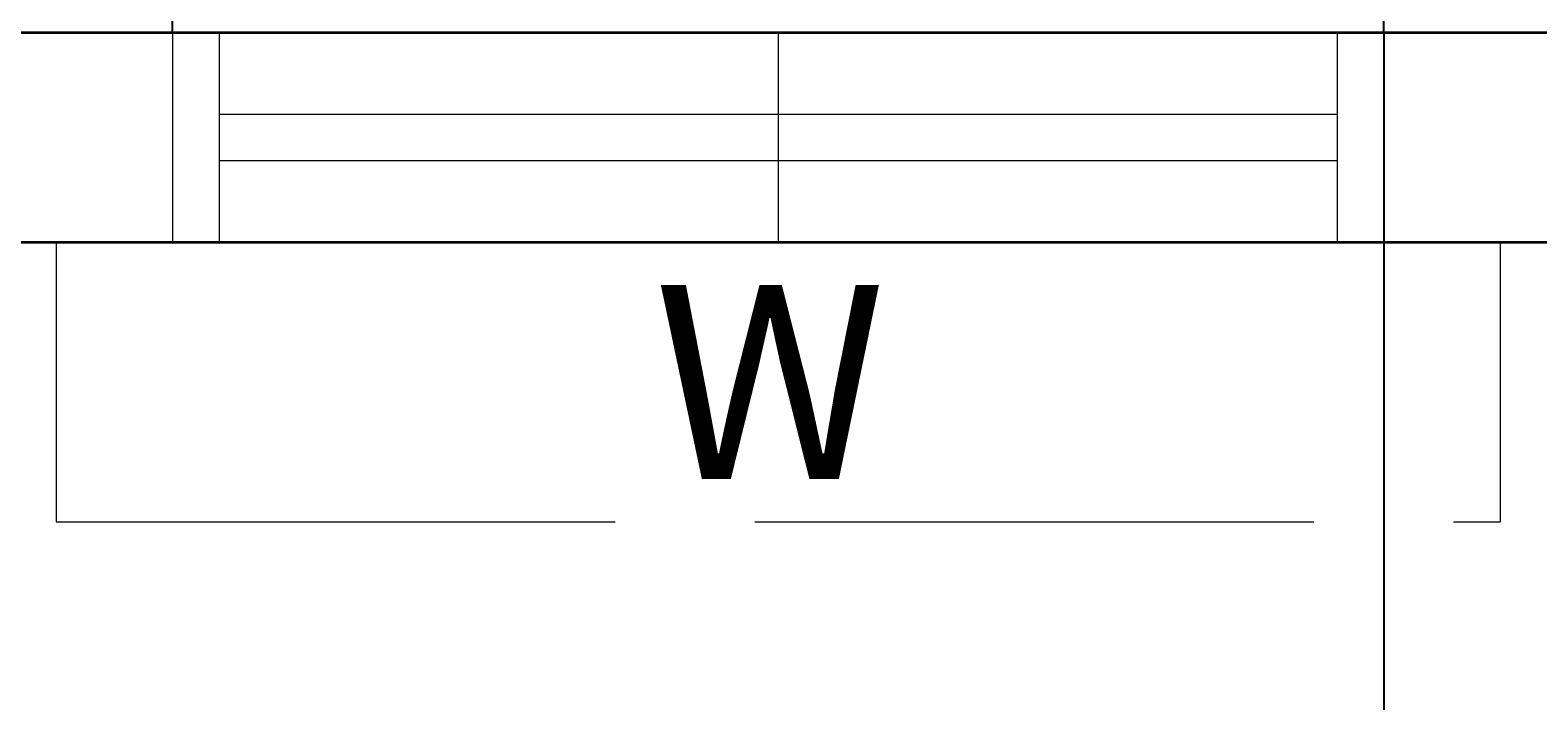
# Model space of a CAD drawing. Units: inches. Extents: x -128 to 854, y -395 to 398.
# Tile 24 of 61: x 199 to 263, y -109 to -80. Entities that reach past the tile are written whole.
import ezdxf

# ---------------------------------------------------------------- set-up
doc = ezdxf.new("R2010")
doc.units = ezdxf.units.IN
doc.header["$MEASUREMENT"] = 0
doc.linetypes.add('ACAD_ISO02W100', pattern=[15, 12, -3])
for name, color, linetype, lineweight in [('A-ANNO-DIMS', 2, 'Continuous', 18), ('A-ANNO-TEXT', 2, 'Continuous', 18), ('A-GLAZ', 220, 'Continuous', 18), ('A-GLAZ-OVHD', 220, 'ACAD_ISO02W100', 13), ('A-WALL', 4, 'Continuous', 35)]:
    doc.layers.add(name, color=color, linetype=linetype, lineweight=lineweight)
doc.styles.get("Standard").update_dxf_attribs({"font": 'arial.ttf'})
doc.dimstyles.get("Standard").update_dxf_attribs({"dimtxt": 0.18, "dimasz": 0.18, "dimexe": 0.18, "dimexo": 0.0625, "dimgap": 0.09, "dimtad": 0, "dimtih": 1, "dimtoh": 1, "dimdec": 1, "dimzin": 0, "dimdsep": 46, "dimlunit": 4, "dimtxsty": 'Standard', "dimcen": 0.09, "dimclrd": 1, "dimclre": 2, "dimclrt": 6, "dimadec": 0, "dimazin": 0, "dimtfac": 1, "dimtdec": 1, "dimtofl": 0, "dimtmove": 0, "dimatfit": 3, "dimfxl": 1, "dimtfill": 2, "dimtfillclr": 3, "dimtolj": 1, "dimtzin": 0, "dimarcsym": 0})

# ---------------------------------------------------------------- blocks, each defined once
blk = doc.blocks.new('*D43')
at = {"layer": 'A-ANNO-DIMS', "color": 0, "lineweight": -2, "transparency": 16777216}
for p, q in [((156.873, -80.197), (156.873, -44.559)), ((304.873, -80.197), (304.873, -44.559)), ((161.873, -44.739), (224.101, -44.739)), ((299.873, -44.739), (237.645, -44.739))]:
    blk.add_line(p, q, dxfattribs=at)
at = {"layer": 'A-ANNO-DIMS', "color": 0, "transparency": 16777216}
for points in [[(161.873, -43.906), (161.873, -45.572), (156.873, -44.739)], [(299.873, -43.906), (299.873, -45.572), (304.873, -44.739)]]:
    blk.add_solid(points, dxfattribs=at)
at = {"layer": 'Defpoints', "color": 0, "transparency": 16777216}
for p in [(304.873, -44.739), (156.873, -80.259), (304.873, -80.259)]:
    blk.add_point(p, dxfattribs=at)
at = {"layer": 'A-ANNO-DIMS', "color": 0, "transparency": 16777216, "insert": (230.873, -44.739), "char_height": 4, "attachment_point": 5, "bg_fill": 1, "box_fill_scale": 1.25, "bg_fill_color": 3, "bg_fill_transparency": 0}
blk.add_mtext('\\A1;12\'-4"', dxfattribs=at)
blk = doc.blocks.new('WIN-48IN')
for p, q in [((9, 52), (0, 52)), ((9, 50), (0, 50)), ((3.5, 50), (3.5, 2)), ((5.5, 50), (5.5, 2)), ((9, 26), (0, 26)), ((9, 2), (0, 2)), ((9, 0), (0, 0))]:
    blk.add_line(p, q)
blk = doc.blocks.new('SHADE-48IN')
at = {"ltscale": 2}
for p, q in [((12, 62), (0, 62)), ((0, 0), (0, 62)), ((12, 57), (12, 62)), ((12, 5), (12, 0)), ((12, 0), (0, 0))]:
    blk.add_line(p, q, dxfattribs=at)
blk = doc.blocks.new('*D71')
at = {"layer": 'A-ANNO-DIMS', "color": 2, "lineweight": -2, "transparency": 16777216}
for p, q in [((204.873, -80.197), (204.873, -72.279)), ((256.873, -80.197), (256.873, -72.279))]:
    blk.add_line(p, q, dxfattribs=at)
at = {"layer": 'A-ANNO-DIMS', "color": 1, "lineweight": -2, "transparency": 16777216}
for p, q in [((205.053, -72.459), (229.644, -72.459)), ((256.693, -72.459), (232.102, -72.459))]:
    blk.add_line(p, q, dxfattribs=at)
at = {"layer": 'A-ANNO-DIMS', "color": 1, "transparency": 16777216}
for points in [[(205.053, -72.429), (205.053, -72.489), (204.873, -72.459)], [(256.693, -72.429), (256.693, -72.489), (256.873, -72.459)]]:
    blk.add_solid(points, dxfattribs=at)
at = {"layer": 'Defpoints', "color": 0, "transparency": 16777216}
for p in [(204.873, -72.459), (204.873, -80.259), (256.873, -80.259)]:
    blk.add_point(p, dxfattribs=at)
at = {"layer": 'A-ANNO-DIMS', "color": 6, "transparency": 16777216, "insert": (230.873, -72.459), "char_height": 0.18, "attachment_point": 5, "bg_fill": 1, "box_fill_scale": 1.25, "bg_fill_color": 3, "bg_fill_transparency": 0}
blk.add_mtext('\\A1;WINDOW 4\'-4" TYP.', dxfattribs=at)
blk = doc.blocks.new('*D72')
at = {"layer": 'A-ANNO-DIMS', "color": 2, "lineweight": -2, "transparency": 16777216}
for p, q in [((256.935, -80.259), (264.853, -80.259)), ((256.935, -89.259), (264.853, -89.259))]:
    blk.add_line(p, q, dxfattribs=at)
at = {"layer": 'A-ANNO-DIMS', "color": 1, "lineweight": -2, "transparency": 16777216}
for p, q in [((264.673, -80.439), (264.673, -84.578)), ((264.673, -89.079), (264.673, -84.941))]:
    blk.add_line(p, q, dxfattribs=at)
at = {"layer": 'A-ANNO-DIMS', "color": 1, "transparency": 16777216}
for points in [[(264.643, -80.439), (264.703, -80.439), (264.673, -80.259)], [(264.643, -89.079), (264.703, -89.079), (264.673, -89.259)]]:
    blk.add_solid(points, dxfattribs=at)
at = {"layer": 'Defpoints', "color": 0, "transparency": 16777216}
for p in [(256.873, -80.259), (264.673, -80.259), (256.873, -89.259)]:
    blk.add_point(p, dxfattribs=at)
at = {"layer": 'A-ANNO-DIMS', "color": 6, "transparency": 16777216, "insert": (264.673, -84.759), "char_height": 0.18, "attachment_point": 5, "bg_fill": 1, "box_fill_scale": 1.25, "bg_fill_color": 3, "bg_fill_transparency": 0}
blk.add_mtext('\\A1;0\'-9" TYP.', dxfattribs=at)
blk = doc.blocks.new('*D114')
at = {"layer": 'A-ANNO-DIMS', "color": 2, "lineweight": -2, "transparency": 16777216}
for p, q in [((256.873, -80.322), (256.873, -127.239)), ((304.873, -80.322), (304.873, -127.239))]:
    blk.add_line(p, q, dxfattribs=at)
at = {"layer": 'A-ANNO-DIMS', "color": 1, "lineweight": -2, "transparency": 16777216}
for p, q in [((257.053, -127.059), (280.54, -127.059)), ((304.693, -127.059), (281.206, -127.059))]:
    blk.add_line(p, q, dxfattribs=at)
at = {"layer": 'A-ANNO-DIMS', "color": 1, "transparency": 16777216}
for points in [[(257.053, -127.029), (257.053, -127.089), (256.873, -127.059)], [(304.693, -127.029), (304.693, -127.089), (304.873, -127.059)]]:
    blk.add_solid(points, dxfattribs=at)
at = {"layer": 'Defpoints', "color": 0, "transparency": 16777216}
for p in [(256.873, -80.259), (304.873, -80.259), (256.873, -127.059)]:
    blk.add_point(p, dxfattribs=at)
at = {"layer": 'A-ANNO-DIMS', "color": 6, "transparency": 16777216, "insert": (280.873, -127.059), "char_height": 0.18, "attachment_point": 5, "bg_fill": 1, "box_fill_scale": 1.25, "bg_fill_color": 3, "bg_fill_transparency": 0}
blk.add_mtext('\\A1;4\'-0"', dxfattribs=at)

msp = doc.modelspace()

# ---------------------------------------------------------------- linework, layer by layer
at = {"layer": 'A-WALL'}
for p, q in [((156.873, -80.259), (304.873, -80.259)), ((156.873, -89.259), (313.873, -89.259))]:
    msp.add_line(p, q, dxfattribs=at)

# ---------------------------------------------------------------- block references
at = {"layer": 'A-GLAZ', "rotation": 90.00000000000006}
msp.add_blockref('WIN-48IN', (256.873, -89.259), dxfattribs=at)
at = {"layer": 'A-GLAZ-OVHD', "extrusion": (0, 0, -1), "zscale": -1, "rotation": 90.00000000000006}
msp.add_blockref('SHADE-48IN', (-199.873, -101.259), dxfattribs=at)

# ---------------------------------------------------------------- texts
at = {"layer": 'A-ANNO-TEXT'}
msp.add_text('W', height=8.314, dxfattribs=at).set_placement((225.543, -99.417))

# ---------------------------------------------------------------- dimensions: what is measured, and where the dimension line sits
at = {"layer": 'A-ANNO-DIMS'}
for base, p1, p2, override, picture, middle in [((304.873, -44.739), (156.873, -80.259), (304.873, -80.259), {"dimtxt": 4, "dimasz": 5, "dimclrd": 0, "dimclre": 0, "dimclrt": 0}, '*D43', (230.873, -44.739)), ((256.873, -127.059), (304.873, -80.259), (256.873, -80.259), {"dimdec": 1, "dimlfac": 1, "dimrnd": 0, "dimzin": 1, "dimdsep": 46, "dimlunit": 4, "dimfrac": 2}, '*D114', (280.873, -127.059))]:
    dim = msp.add_linear_dim(base=base, p1=p1, p2=p2, dimstyle='Standard', override=override, dxfattribs=at)
    dim.commit()
    dim.dimension.update_dxf_attribs({"geometry": picture, "text_midpoint": middle})
for base, p1, p2, angle, text, picture, middle in [((204.873, -72.459), (256.873, -80.259), (204.873, -80.259), 180, 'WINDOW <> TYP.', '*D71', (230.873, -72.459)), ((264.673, -80.259), (256.873, -89.259), (256.873, -80.259), 90, '<> TYP.', '*D72', (264.673, -84.759))]:
    dim = msp.add_linear_dim(base=base, p1=p1, p2=p2, angle=angle, text=text, dimstyle='Standard', override={"dimdec": 1, "dimlfac": 1, "dimrnd": 0, "dimzin": 1, "dimdsep": 46, "dimlunit": 4, "dimfrac": 2}, dxfattribs=at)
    dim.commit()
    dim.dimension.update_dxf_attribs({"geometry": picture, "text_midpoint": middle})

doc.saveas('drawing.dxf')
